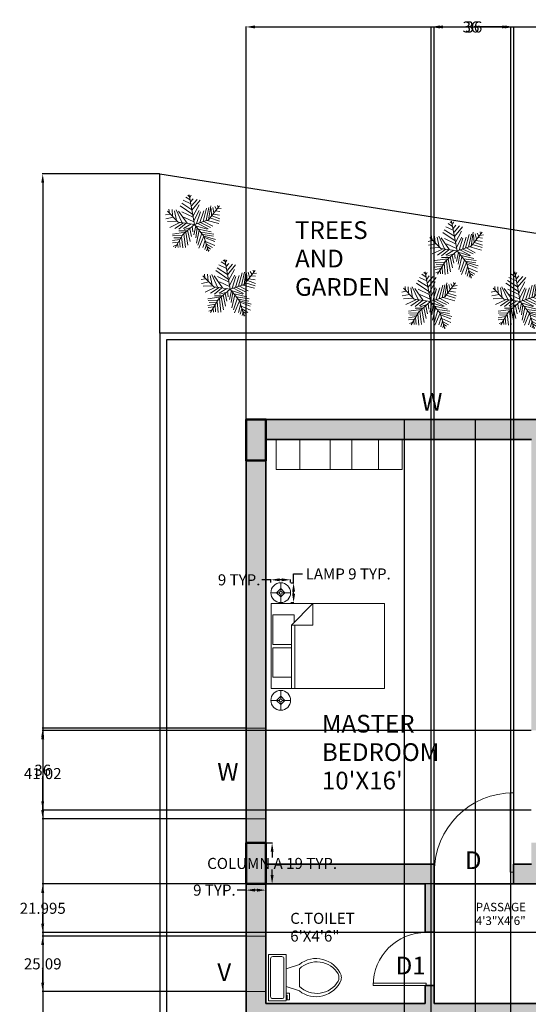
# Model space of a CAD drawing. Units: inches. Extents: x 460 to 1030, y -658 to 271.
# Tile 7 of 10: x 460 to 690, y -174 to 271. Entities that reach past the tile are written whole.
import ezdxf

# ---------------------------------------------------------------- set-up
doc = ezdxf.new("R2010")
doc.units = ezdxf.units.IN
doc.header["$MEASUREMENT"] = 0
for name, color, linetype, lineweight in [('A-ANNO-DIMS', 2, 'Continuous', 18), ('A-ANNO-TEXT', 7, 'Continuous', 18), ('A-AREA-IDEN', 7, 'Continuous', 25), ('A-COLS', 7, 'Continuous', 50), ('A-DOOR', 3, 'Continuous', 20), ('A-FLOR-CASE', 9, 'Continuous', 18), ('A-FLOR-FIXT', 9, 'Continuous', 18), ('A-FURN', 8, 'Continuous', 18), ('A-GLAZ', 4, 'Continuous', 20), ('A-GLAZ-PATT', 4, 'Continuous', 13), ('A-WALL', 7, 'Continuous', 35), ('A-WALL-PATT', 5, 'Continuous', 13), ('C-ANNO-TEXT', 7, 'Continuous', 18), ('C-PROP', 7, 'Continuous', 25), ('L-PLNT', 94, 'Continuous', 13)]:
    doc.layers.add(name, color=color, linetype=linetype, lineweight=lineweight)
doc.layers.add('A-COLS-PATT', color=7, linetype='Continuous', lineweight=13, true_color=0xffffff)
doc.styles.get("Standard").update_dxf_attribs({"font": 'arial.ttf'})
doc.dimstyles.get("Standard").update_dxf_attribs({"dimtxt": 5, "dimasz": 4, "dimexe": 0.18, "dimexo": 0.0625, "dimgap": 0.09, "dimtad": 0, "dimtih": 1, "dimtoh": 1, "dimdec": 1, "dimzin": 0, "dimdsep": 46, "dimlunit": 4, "dimtxsty": 'Standard', "dimcen": 0.09, "dimadec": 0, "dimazin": 0, "dimtfac": 1, "dimtdec": 1, "dimtofl": 0, "dimtmove": 0, "dimatfit": 3, "dimfxl": 1, "dimtolj": 1, "dimtzin": 0, "dimarcsym": 0})

# ---------------------------------------------------------------- blocks, each defined once
blk = doc.blocks.new('Bed - Queen')
for p, q in [((0, -80.00003), (0, 0)), ((0, 0), (59.99999, 0)), ((59.99999, 0), (59.99999, -80.00003)), ((7.99999, -1.2), (28.79998, -1.2)), ((7.99999, -14.4), (7.99999, -1.2)), ((28.79998, -1.2), (28.79998, -14.4)), ((31.19999, -1.2), (51.99999, -1.2)), ((31.19999, -14.4), (31.19999, -1.2)), ((51.99999, -1.2), (51.99999, -16.4)), ((0, -14.4), (44.8, -14.4)), ((44.8, -16.8), (0, -16.8)), ((59.99999, -29.6), (44.8, -14.4)), ((44.8, -14.4), (44.8, -29.6)), ((51.99999, -16.4), (46.79936, -16.4)), ((44.8, -29.6), (59.99999, -29.6)), ((59.99999, -80.00003), (0, -80.00003))]:
    blk.add_line(p, q)
blk = doc.blocks.new('Lamp - Table')
for p, q in [((0, 7), (0, 1)), ((-1, 0), (-7, 0)), ((0, 3), (-3, 0)), ((-3, 0), (0, -3)), ((3, 0), (0, 3)), ((0, -3), (3, 0)), ((1, 0), (7, 0)), ((0, -1), (0, -7))]:
    blk.add_line(p, q)
for radius in [7, 1]:
    blk.add_circle((0, 0), radius)
blk = doc.blocks.new('*U2')
for p, q in [((0, 0), (0, -6)), ((40, 0), (40, -6))]:
    blk.add_line(p, q)
blk.add_lwpolyline([(0, 0), (0, 40), (1.75, 40), (1.75, 0)], close=True)
blk.add_arc((0, 0), 40, 0, 90)
blk = doc.blocks.new('*U4')
for p, q in [((9.5, -6), (9.5, -2)), ((-10, -8.5), (-8, -8.5)), ((-10, -9.5), (-10, -8.5)), ((-8, -8.5), (-8, -8)), ((-7, -8), (-7, -9.5)), ((-4, -8), (-6, -14)), ((4, -8), (6, -14)), ((-7, -9.5), (-10, -9.5)), ((4, -14), (-4, -14))]:
    blk.add_line(p, q)
blk.add_lwpolyline([(10.5, -8), (10.5, 0), (-10.5, 0), (-10.5, -8)], close=True)
for points in [[(-9.5, -2), (-9.5, -6)], [(8.5, -1), (-8.5, -1)], [(-8.5, -7), (8.5, -7)]]:
    blk.add_lwpolyline(points)
for centre, radius, start, end in [((-8.62, -1.88), 0.884, 81.8699, 188.1301), ((8.62, -1.88), 0.884, 351.8699, 98.1301), ((-8.62, -6.12), 0.884, 171.8699, 278.1301), ((8.62, -6.12), 0.884, 261.8699, 8.1301), ((3.52, -21.58), 12.17, 141.4691, 247.9714), ((4.2, -21.82), 11.33, 136.3677, 238.9468), ((-3.52, -21.58), 12.17, 292.0284, 38.5307), ((-4.2, -21.82), 11.33, 301.053, 43.6321), ((0, -27.88), 4, 245.7318, 294.2682), ((0, -29), 4, 254.8605, 285.1395)]:
    blk.add_arc(centre, radius, start, end)
blk = doc.blocks.new('*U11')
for p, q in [((0, 0), (-266.7, 1447.8)), ((-129.8956, 713.6638), (-626.7704, 1032.1544)), ((-185.1152, 1008.5578), (-553.1612, 1185.4942)), ((-221.9198, 1197.3052), (-433.5526, 1338.8594)), ((-258.7244, 1362.456), (-332.3336, 1421.4348)), ((-231.1146, 1315.2628), (-166.7002, 1421.4348)), ((-194.31, 1102.9442), (-65.4812, 1256.284)), ((-148.3106, 914.1968), (118.5418, 1220.9018)), ((-129.8956, 701.8528), (265.7602, 1185.4942)), ((-1206.4492, 501.3198), (-1418.082, 465.9376)), ((-800.1, 114.3), (-1333.5, 647.7)), ((-1234.059, 536.7274), (-1252.4486, 737.2604)), ((-1105.2302, 725.4494), (-1077.6458, 395.1732)), ((-976.4268, 666.4706), (-884.4026, 194.6402)), ((-902.8176, 713.6638), (-617.5756, 100.2538)), ((-369.1382, 53.086), (-783.1836, 642.874)), ((-93.091, 489.5342), (-700.3796, 902.3858)), ((-617.5756, 607.4918), (-74.7014, 347.98)), ((-74.7014, 418.7444), (219.7608, 961.39)), ((-28.6766, 171.0436), (228.9556, 678.2816)), ((100.1268, 41.275), (284.1498, 619.2774)), ((256.5654, 88.4682), (449.7832, 666.4706)), ((412.9786, 147.447), (587.8068, 796.2392)), ((560.197, 182.8292), (698.2206, 819.8358)), ((685.8, 228.6), (1219.2, 914.4)), ((689.0258, 230.0224), (790.2448, 914.1968)), ((808.6344, 784.4282), (827.0494, 418.7444)), ((891.4384, 831.6214), (946.658, 572.1096)), ((919.0482, 501.3198), (1222.6798, 454.152)), ((983.4626, 867.0036), (1066.2666, 725.4494)), ((1029.462, 654.685), (1241.0948, 631.0884)), ((1112.2914, 760.8316), (1296.3144, 784.4282)), ((1121.4862, 925.9824), (1149.0706, 831.6214)), ((-1031.621, 347.98), (-1399.667, 277.1902)), ((-847.598, 159.2326), (-1326.0578, 135.636)), ((-718.7946, 88.4682), (-1215.644, -147.447)), ((-543.9664, 76.6572), (-967.2066, -206.4512)), ((0, 0), (-800.1, 114.3)), ((-405.9428, 53.086), (-764.794, -241.8334)), ((0, 0), (-571.5, -495.3)), ((-166.7002, 29.4894), (-543.9664, -206.4512)), ((-525.5514, 347.98), (-28.6766, 123.8504)), ((0, 0), (685.8, 228.6)), ((0, 0), (457.2, -571.5)), ((164.5412, 41.275), (661.416, -218.2368)), ((284.1498, 88.4682), (781.0246, -147.447)), ((458.978, 147.447), (891.4384, -88.4682)), ((615.4166, 194.6402), (1185.8752, 41.275)), ((753.4148, 312.5978), (1222.6798, 159.2326)), ((845.439, 418.7444), (1241.0948, 277.1902)), ((-442.7474, -383.3876), (-1086.8406, -477.7486)), ((-387.5278, -324.4088), (-764.794, -324.4088)), ((-525.5514, -465.963), (-451.9422, -1126.5408)), ((-166.7002, -147.447), (-507.1618, -253.619)), ((-433.5526, -383.3876), (-323.1134, -1020.3688)), ((-341.5284, -289.0012), (-221.9198, -831.6214)), ((-240.3094, -218.2368), (-157.5054, -595.7062)), ((-120.7008, -88.4682), (-93.091, -371.5766)), ((63.3222, -76.6826), (-37.8714, -513.1308)), ((44.9326, -64.897), (615.4166, -241.8334)), ((127.7366, -159.258), (54.1274, -654.685)), ((228.9556, -289.0012), (90.932, -914.1968)), ((357.759, -430.5554), (164.5412, -1020.3688)), ((192.151, -230.0224), (817.8292, -371.5766)), ((311.7596, -383.3876), (937.4378, -477.7486)), ((-718.7946, -737.2604), (-1086.8406, -796.2392)), ((-617.5756, -548.5384), (-1077.6458, -560.324)), ((-783.1836, -867.029), (-1077.6458, -902.4112)), ((-681.9646, -666.496), (-1022.4262, -654.685)), ((-571.5, -495.3), (-952.5, -1143)), ((-829.2084, -937.7934), (-810.7934, -1126.5408)), ((-737.1842, -784.4536), (-709.5744, -1114.7298)), ((-635.9652, -607.5172), (-580.771, -1150.1374)), ((458.978, -572.1096), (210.5406, -1161.923)), ((514.1976, -772.6426), (403.7838, -1138.3264)), ((412.9786, -501.3452), (919.0482, -583.9206)), ((457.2, -571.5), (685.8, -1333.5)), ((468.1982, -572.1096), (1029.462, -737.2604)), ((486.5878, -642.8994), (983.4626, -843.4324)), ((578.612, -961.39), (495.7826, -1232.7128)), ((541.8074, -831.6214), (992.6574, -1032.1544)), ((-875.2078, -1008.5832), (-1040.8412, -1079.3476)), ((578.612, -973.1756), (873.0488, -1138.3264)), ((624.6114, -1161.923), (587.8068, -1291.6916)), ((624.6114, -1102.9442), (781.0246, -1209.1162)), ((679.8056, -1268.095), (716.6102, -1291.6916))]:
    blk.add_line(p, q)
blk = doc.blocks.new('BEDROOM-STORAGE-UNIT')
for p, q in [((10.68, 0), (10.68, -13.59)), ((24.45, 0), (24.45, -13.59)), ((34.21, 0), (34.21, -13.59)), ((46.22, 0), (46.22, -13.59))]:
    blk.add_line(p, q)
blk.add_lwpolyline([(0, 0), (57.01, 0), (57.01, -13.59), (0, -13.59)], close=True)
blk = doc.blocks.new('COL-RECT-TYPE-A')
blk.add_lwpolyline([(0, 0), (9, 0), (9, -18.58), (0, -18.58)], close=True)
blk = doc.blocks.new('*D19')
at = {"layer": 'A-ANNO-DIMS', "color": 0, "lineweight": -2, "transparency": 16777216}
for p, q in [((571.86, -101.15), (574.76, -101.15)), ((574.58, -105.15), (574.58, -107.76)), ((574.58, -115.73), (574.58, -113.11)), ((571.86, -119.73), (574.76, -119.73))]:
    blk.add_line(p, q, dxfattribs=at)
at = {"layer": 'A-ANNO-DIMS', "color": 0, "transparency": 16777216}
for points in [[(573.92, -105.15), (575.25, -105.15), (574.58, -101.15)], [(573.92, -115.73), (575.25, -115.73), (574.58, -119.73)]]:
    blk.add_solid(points, dxfattribs=at)
at = {"layer": 'Defpoints', "color": 0, "transparency": 16777216}
for p in [(571.8, -101.15), (571.8, -119.73), (574.58, -119.73)]:
    blk.add_point(p, dxfattribs=at)
at = {"layer": 'A-ANNO-DIMS', "color": 0, "transparency": 16777216, "insert": (574.58, -110.44), "char_height": 5, "attachment_point": 5}
blk.add_mtext('\\A1;COLUMN A 19 TYP.', dxfattribs=at)
blk = doc.blocks.new('*D20')
at = {"layer": 'A-ANNO-DIMS', "color": 0, "lineweight": -2, "transparency": 16777216}
for p, q in [((562.8, -119.79), (562.8, -122.69)), ((571.8, -119.79), (571.8, -122.69)), ((562.8, -122.51), (558.8, -122.51)), ((567.8, -122.51), (566.8, -122.51))]:
    blk.add_line(p, q, dxfattribs=at)
at = {"layer": 'A-ANNO-DIMS', "color": 0, "transparency": 16777216}
for points in [[(566.8, -121.85), (566.8, -123.18), (562.8, -122.51)], [(567.8, -121.85), (567.8, -123.18), (571.8, -122.51)]]:
    blk.add_solid(points, dxfattribs=at)
at = {"layer": 'Defpoints', "color": 0, "transparency": 16777216}
for p in [(562.8, -119.73), (571.8, -119.73), (562.8, -122.51)]:
    blk.add_point(p, dxfattribs=at)
at = {"layer": 'A-ANNO-DIMS', "color": 0, "transparency": 16777216, "insert": (548.48, -122.51), "char_height": 5, "attachment_point": 5}
blk.add_mtext('\\A1;9 TYP.', dxfattribs=at)
blk = doc.blocks.new('*D23')
at = {"layer": 'A-ANNO-DIMS', "color": 0, "lineweight": -2, "transparency": 16777216}
for p, q in [((584.29, 16.44), (584.29, 20.44)), ((584.29, 20.44), (588.29, 20.44)), ((583.01, 16.44), (584.47, 16.44)), ((584.29, 11.48), (584.29, 12.44)), ((583.01, 7.48), (584.47, 7.48))]:
    blk.add_line(p, q, dxfattribs=at)
at = {"layer": 'A-ANNO-DIMS', "color": 0, "transparency": 16777216}
for points in [[(583.63, 12.44), (584.96, 12.44), (584.29, 16.44)], [(583.63, 11.48), (584.96, 11.48), (584.29, 7.48)]]:
    blk.add_solid(points, dxfattribs=at)
at = {"layer": 'Defpoints', "color": 0, "transparency": 16777216}
for p in [(582.95, 16.44), (584.29, 16.44), (582.95, 7.48)]:
    blk.add_point(p, dxfattribs=at)
at = {"layer": 'A-ANNO-DIMS', "color": 0, "transparency": 16777216, "insert": (608.98, 20.44), "char_height": 5, "attachment_point": 5}
blk.add_mtext('\\A1;LAMP 9 TYP.', dxfattribs=at)
blk = doc.blocks.new('*D24')
at = {"layer": 'A-ANNO-DIMS', "color": 0, "lineweight": -2, "transparency": 16777216}
for p, q in [((573.99, 16.5), (573.99, 17.96)), ((582.95, 16.5), (582.95, 17.96)), ((573.99, 17.78), (569.99, 17.78)), ((578.95, 17.78), (577.99, 17.78))]:
    blk.add_line(p, q, dxfattribs=at)
at = {"layer": 'A-ANNO-DIMS', "color": 0, "transparency": 16777216}
for points in [[(577.99, 18.45), (577.99, 17.12), (573.99, 17.78)], [(578.95, 18.45), (578.95, 17.12), (582.95, 17.78)]]:
    blk.add_solid(points, dxfattribs=at)
at = {"layer": 'Defpoints', "color": 0, "transparency": 16777216}
for p in [(573.99, 17.78), (573.99, 16.44), (582.95, 16.44)]:
    blk.add_point(p, dxfattribs=at)
at = {"layer": 'A-ANNO-DIMS', "color": 0, "transparency": 16777216, "insert": (559.67, 17.78), "char_height": 5, "attachment_point": 5}
blk.add_mtext('\\A1;9 TYP.', dxfattribs=at)
blk = doc.blocks.new('*D40')
at = {"layer": 'A-ANNO-DIMS', "color": 0, "lineweight": -2, "transparency": 16777216}
for p, q in [((523.73, 201.27), (470.68, 201.27)), ((470.86, 197.27), (470.86, -202.58)), ((470.86, -607.73), (470.86, -207.87)), ((523.73, -611.73), (470.68, -611.73))]:
    blk.add_line(p, q, dxfattribs=at)
at = {"layer": 'A-ANNO-DIMS', "color": 0, "transparency": 16777216}
for points in [[(470.19, 197.27), (471.52, 197.27), (470.86, 201.27)], [(470.19, -607.73), (471.52, -607.73), (470.86, -611.73)]]:
    blk.add_solid(points, dxfattribs=at)
at = {"layer": 'Defpoints', "color": 0, "transparency": 16777216}
for p in [(470.86, 201.27), (523.8, 201.27), (523.8, -611.73)]:
    blk.add_point(p, dxfattribs=at)
at = {"layer": 'A-ANNO-DIMS', "color": 0, "transparency": 16777216, "insert": (470.86, -205.23), "char_height": 5, "attachment_point": 5}
blk.add_mtext('\\A1;813', dxfattribs=at)
blk = doc.blocks.new('*D43')
at = {"layer": 'A-ANNO-DIMS', "color": 0, "lineweight": -2, "transparency": 16777216}
for p, q in [((562.8, 90.34), (562.8, 267.89)), ((566.8, 267.71), (746.18, 267.71)), ((936.8, 267.71), (757.41, 267.71)), ((940.8, 90.34), (940.8, 267.89))]:
    blk.add_line(p, q, dxfattribs=at)
at = {"layer": 'A-ANNO-DIMS', "color": 0, "transparency": 16777216}
for points in [[(566.8, 268.38), (566.8, 267.04), (562.8, 267.71)], [(936.8, 268.38), (936.8, 267.04), (940.8, 267.71)]]:
    blk.add_solid(points, dxfattribs=at)
at = {"layer": 'Defpoints', "color": 0, "transparency": 16777216}
for p in [(940.8, 267.71), (562.8, 90.27), (940.8, 90.27)]:
    blk.add_point(p, dxfattribs=at)
at = {"layer": 'A-ANNO-DIMS', "color": 0, "transparency": 16777216, "insert": (751.8, 267.71), "char_height": 5, "attachment_point": 5}
blk.add_mtext('\\A1;378', dxfattribs=at)
blk = doc.blocks.new('*D55')
at = {"layer": 'A-ANNO-DIMS', "color": 0, "lineweight": -2, "transparency": 16777216}
for p, q in [((894.56, -119.73), (470.68, -119.73)), ((470.86, -123.73), (470.86, -128.08)), ((470.86, -137.72), (470.86, -133.37)), ((894.55, -141.72), (470.68, -141.72))]:
    blk.add_line(p, q, dxfattribs=at)
at = {"layer": 'A-ANNO-DIMS', "color": 0, "transparency": 16777216}
for points in [[(470.19, -123.73), (471.52, -123.73), (470.86, -119.73)], [(470.19, -137.72), (471.52, -137.72), (470.86, -141.72)]]:
    blk.add_solid(points, dxfattribs=at)
at = {"layer": 'Defpoints', "color": 0, "transparency": 16777216}
for p in [(470.86, -119.73), (894.62, -119.73), (894.61, -141.72)]:
    blk.add_point(p, dxfattribs=at)
at = {"layer": 'A-ANNO-DIMS', "color": 0, "transparency": 16777216, "insert": (470.86, -130.72), "char_height": 5, "attachment_point": 5}
blk.add_mtext('\\A1;21.995', dxfattribs=at)
blk = doc.blocks.new('*D56')
at = {"layer": 'A-ANNO-DIMS', "color": 0, "lineweight": -2, "transparency": 16777216}
for p, q in [((647.8, -110.66), (647.8, 267.89)), ((651.8, 267.71), (662.13, 267.71)), ((679.8, 267.71), (669.46, 267.71)), ((683.8, -110.66), (683.8, 267.89))]:
    blk.add_line(p, q, dxfattribs=at)
at = {"layer": 'A-ANNO-DIMS', "color": 0, "transparency": 16777216}
for points in [[(651.8, 268.38), (651.8, 267.04), (647.8, 267.71)], [(679.8, 268.38), (679.8, 267.04), (683.8, 267.71)]]:
    blk.add_solid(points, dxfattribs=at)
at = {"layer": 'Defpoints', "color": 0, "transparency": 16777216}
for p in [(683.8, 267.71), (647.8, -110.73), (683.8, -110.73)]:
    blk.add_point(p, dxfattribs=at)
at = {"layer": 'A-ANNO-DIMS', "color": 0, "transparency": 16777216, "insert": (665.8, 267.71), "char_height": 5, "attachment_point": 5}
blk.add_mtext('\\A1;36', dxfattribs=at)
blk = doc.blocks.new('*D58')
at = {"layer": 'A-ANNO-DIMS', "color": 0, "lineweight": -2, "transparency": 16777216}
for p, q in [((691.73, -50.3), (470.68, -50.3)), ((470.86, -54.3), (470.86, -65.65)), ((470.86, -82.3), (470.86, -70.94)), ((691.73, -86.3), (470.68, -86.3))]:
    blk.add_line(p, q, dxfattribs=at)
at = {"layer": 'A-ANNO-DIMS', "color": 0, "transparency": 16777216}
for points in [[(470.19, -54.3), (471.52, -54.3), (470.86, -50.3)], [(470.19, -82.3), (471.52, -82.3), (470.86, -86.3)]]:
    blk.add_solid(points, dxfattribs=at)
at = {"layer": 'Defpoints', "color": 0, "transparency": 16777216}
for p in [(691.8, -50.3), (470.86, -86.3), (691.8, -86.3)]:
    blk.add_point(p, dxfattribs=at)
at = {"layer": 'A-ANNO-DIMS', "color": 0, "transparency": 16777216, "insert": (470.86, -68.3), "char_height": 5, "attachment_point": 5}
blk.add_mtext('\\A1;36', dxfattribs=at)
blk = doc.blocks.new('*D61')
at = {"layer": 'A-ANNO-DIMS', "color": 0, "lineweight": -2, "transparency": 16777216}
for p, q in [((646.47, -287.66), (646.47, 267.89)), ((650.47, 267.71), (660.81, 267.71)), ((678.47, 267.71), (668.14, 267.71)), ((682.47, -287.66), (682.47, 267.89))]:
    blk.add_line(p, q, dxfattribs=at)
at = {"layer": 'A-ANNO-DIMS', "color": 0, "transparency": 16777216}
for points in [[(650.47, 268.38), (650.47, 267.04), (646.47, 267.71)], [(678.47, 268.38), (678.47, 267.04), (682.47, 267.71)]]:
    blk.add_solid(points, dxfattribs=at)
at = {"layer": 'Defpoints', "color": 0, "transparency": 16777216}
for p in [(682.47, 267.71), (646.47, -287.73), (682.47, -287.73)]:
    blk.add_point(p, dxfattribs=at)
at = {"layer": 'A-ANNO-DIMS', "color": 0, "transparency": 16777216, "insert": (664.47, 267.71), "char_height": 5, "attachment_point": 5}
blk.add_mtext('\\A1;36', dxfattribs=at)
blk = doc.blocks.new('*D68')
at = {"layer": 'A-ANNO-DIMS', "color": 0, "lineweight": -2, "transparency": 16777216}
for p, q in [((634.27, 90.21), (634.27, -654.61)), ((666.46, 90.21), (666.46, -654.61)), ((638.27, -654.43), (639.91, -654.43)), ((662.46, -654.43), (660.82, -654.43))]:
    blk.add_line(p, q, dxfattribs=at)
at = {"layer": 'A-ANNO-DIMS', "color": 0, "transparency": 16777216}
for points in [[(638.27, -653.77), (638.27, -655.1), (634.27, -654.43)], [(662.46, -653.77), (662.46, -655.1), (666.46, -654.43)]]:
    blk.add_solid(points, dxfattribs=at)
at = {"layer": 'Defpoints', "color": 0, "transparency": 16777216}
for p in [(634.27, 90.27), (666.46, 90.27), (666.46, -654.43)]:
    blk.add_point(p, dxfattribs=at)
at = {"layer": 'A-ANNO-DIMS', "color": 0, "transparency": 16777216, "insert": (650.37, -654.43), "char_height": 5, "attachment_point": 5}
blk.add_mtext('\\A1;32.184', dxfattribs=at)
blk = doc.blocks.new('*D74')
at = {"layer": 'A-ANNO-DIMS', "color": 0, "lineweight": -2, "transparency": 16777216}
for p, q in [((562.73, -49.3), (470.68, -49.3)), ((470.86, -53.3), (470.86, -67.17)), ((470.86, -86.32), (470.86, -72.45)), ((562.73, -90.32), (470.68, -90.32))]:
    blk.add_line(p, q, dxfattribs=at)
at = {"layer": 'A-ANNO-DIMS', "color": 0, "transparency": 16777216}
for points in [[(470.19, -53.3), (471.52, -53.3), (470.86, -49.3)], [(470.19, -86.32), (471.52, -86.32), (470.86, -90.32)]]:
    blk.add_solid(points, dxfattribs=at)
at = {"layer": 'Defpoints', "color": 0, "transparency": 16777216}
for p in [(562.8, -49.3), (470.86, -90.32), (562.8, -90.32)]:
    blk.add_point(p, dxfattribs=at)
at = {"layer": 'A-ANNO-DIMS', "color": 0, "transparency": 16777216, "insert": (470.86, -69.81), "char_height": 5, "attachment_point": 5}
blk.add_mtext('\\A1;41.02', dxfattribs=at)
blk = doc.blocks.new('*D75')
at = {"layer": 'A-ANNO-DIMS', "color": 0, "lineweight": -2, "transparency": 16777216}
for p, q in [((562.73, -143.29), (470.68, -143.29)), ((470.86, -147.29), (470.86, -153.19)), ((470.86, -164.38), (470.86, -158.48)), ((562.73, -168.38), (470.68, -168.38))]:
    blk.add_line(p, q, dxfattribs=at)
at = {"layer": 'A-ANNO-DIMS', "color": 0, "transparency": 16777216}
for points in [[(470.19, -147.29), (471.52, -147.29), (470.86, -143.29)], [(470.19, -164.38), (471.52, -164.38), (470.86, -168.38)]]:
    blk.add_solid(points, dxfattribs=at)
at = {"layer": 'Defpoints', "color": 0, "transparency": 16777216}
for p in [(562.8, -143.29), (470.86, -168.38), (562.8, -168.38)]:
    blk.add_point(p, dxfattribs=at)
at = {"layer": 'A-ANNO-DIMS', "color": 0, "transparency": 16777216, "insert": (470.86, -155.83), "char_height": 5, "attachment_point": 5}
blk.add_mtext('\\A1;25.09', dxfattribs=at)

msp = doc.modelspace()

# ---------------------------------------------------------------- hatches: boundary and pattern name
at = {"layer": 'A-COLS-PATT'}
h = msp.add_hatch(color=256, dxfattribs=at)
h.dxf.hatch_style = 1
h.paths.add_polyline_path([(571.7961, 90.2738), (562.7961, 90.2738), (562.7961, 71.6966), (571.7961, 71.6966)])
h.paths.add_polyline_path([(700.7961, 90.2738), (691.7961, 90.2738), (691.7961, 71.6966), (700.7961, 71.6966)])
h.paths.add_polyline_path([(811.7961, 90.2738), (802.7961, 90.2738), (802.7961, 71.6966), (811.7961, 71.6966)])
h.paths.add_polyline_path([(940.7961, 90.2738), (931.7961, 90.2738), (931.7961, 71.6966), (940.7961, 71.6966)])
h.paths.add_polyline_path([(940.7961, -101.149), (931.7961, -101.149), (931.7961, -119.7262), (940.7961, -119.7262)])
h.paths.add_polyline_path([(940.7961, -268.3723), (931.7961, -268.3723), (931.7961, -287.7262), (940.7961, -287.7262)])
h.paths.add_polyline_path([(803.0275, -281.7262), (789.8237, -281.7262), (789.8237, -287.7262), (803.0275, -287.7262)])
h.paths.add_polyline_path([(700.7961, -303.809), (691.7961, -303.809), (691.7961, -323.8443), (700.7961, -323.8443)])
h.paths.add_polyline_path([(571.7961, -303.809), (562.7961, -303.809), (562.7961, -323.8443), (571.7961, -323.8443)])
h.paths.add_polyline_path([(571.7961, -413.1453), (562.7961, -413.1453), (562.7961, -432.4659), (571.7961, -432.4659)])
h.paths.add_polyline_path([(571.7961, -101.149), (562.7961, -101.149), (562.7961, -119.7262), (571.7961, -119.7262)])
h.paths.add_polyline_path([(700.7961, -101.0985), (691.7961, -101.0985), (691.7961, -119.7262), (700.7961, -119.7262)])
h.paths.add_polyline_path([(811.7961, -101.149), (802.7961, -101.149), (802.7961, -119.7262), (811.7961, -119.7262)])
at = {"layer": 'A-GLAZ-PATT'}
h = msp.add_hatch(color=256, dxfattribs=at)
h.dxf.hatch_style = 1
h.paths.add_polyline_path([(571.7961, -343.9041), (562.7961, -343.9041), (562.7961, -384.3969), (571.7961, -384.3969)])
h.paths.add_polyline_path([(571.7961, -143.2895), (562.7961, -143.2895), (562.7961, -168.3798), (571.7961, -168.3798)])
h.paths.add_polyline_path([(571.7961, -49.2966), (562.7961, -49.2966), (562.7961, -90.3192), (571.7961, -90.3192)])
h.paths.add_polyline_path([(666.4584, 90.2738), (634.2742, 90.2738), (634.2742, 81.2738), (666.4584, 81.2738)])
h.paths.add_polyline_path([(742.1779, 90.2738), (713.201, 90.2738), (713.201, 81.2738), (742.1779, 81.2738)])
h.paths.add_polyline_path([(797.2395, 90.2738), (768.2626, 90.2738), (768.2626, 81.2738), (797.2395, 81.2738)])
h.paths.add_polyline_path([(918.7723, 90.2738), (881.2728, 90.2738), (881.2728, 81.2738), (918.7723, 81.2738)])
h.paths.add_polyline_path([(940.7961, -60.0042), (931.7961, -60.0042), (931.7961, -95.7262), (940.7961, -95.7262)])
h.paths.add_polyline_path([(940.7961, -163.6558), (931.7961, -163.6558), (931.7961, -230.2946), (940.7961, -230.2946)])
h.paths.add_polyline_path([(913.7961, -331.7262), (835.7961, -331.7262), (835.7961, -332.7262), (913.7961, -332.7262)])
h.paths.add_polyline_path([(871.4559, -281.7262), (831.4302, -281.7262), (831.4302, -287.7262), (871.4559, -287.7262)])
h.paths.add_polyline_path([(774.8576, -281.7262), (716.7073, -281.7262), (716.7073, -287.7262), (774.8576, -287.7262)])
at = {"layer": 'A-WALL-PATT'}
h = msp.add_hatch(color=256, dxfattribs=at)
h.dxf.hatch_style = 1
h.paths.add_polyline_path([(634.2742, 90.2738), (571.7961, 90.2738), (571.7961, 81.2738), (634.2742, 81.2738)])
h.paths.add_polyline_path([(691.7961, 90.2738), (666.4584, 90.2738), (666.4584, 81.2738), (691.7961, 81.2738)])
h.paths.add_polyline_path([(713.201, 90.2738), (700.7961, 90.2738), (700.7961, 81.2738), (713.201, 81.2738)])
h.paths.add_polyline_path([(748.7961, 90.2738), (742.1779, 90.2738), (742.1779, 81.2738), (748.7961, 81.2738)])
h.paths.add_polyline_path([(768.2626, 90.2738), (754.7961, 90.2738), (754.7961, 81.2738), (768.2626, 81.2738)])
h.paths.add_polyline_path([(802.7961, 90.2738), (797.2395, 90.2738), (797.2395, 81.2738), (802.7961, 81.2738)])
h.paths.add_polyline_path([(881.2728, 90.2738), (811.7961, 90.2738), (811.7961, 81.2738), (881.2728, 81.2738)])
h.paths.add_polyline_path([(931.7961, 90.2738), (918.7723, 90.2738), (918.7723, 81.2738), (931.7961, 81.2738)])
h.paths.add_polyline_path([(940.7961, 71.6966), (931.7961, 71.6966), (931.7961, -60.0042), (940.7961, -60.0042)])
h.paths.add_polyline_path([(940.7961, -95.7262), (931.7961, -95.7262), (931.7961, -101.149), (940.7961, -101.149)])
h.paths.add_polyline_path([(931.7961, -110.7262), (894.6225, -110.7262), (894.6225, -119.7262), (931.7961, -119.7262)])
h.paths.add_polyline_path([(858.6225, -110.7262), (811.7961, -110.7262), (811.7961, -119.7262), (858.6225, -119.7262)])
h.paths.add_polyline_path([(940.7961, -119.7262), (931.7961, -119.7262), (931.7961, -141.7212), (931.7961, -163.6558), (940.7961, -163.6558)])
h.paths.add_polyline_path([(940.7961, -230.2946), (931.7961, -230.2946), (931.7961, -268.3723), (940.7961, -268.3723)])
h.paths.add_polyline_path([(931.7961, -281.7262), (908.3452, -281.7262), (908.3452, -285.0181), (908.3452, -287.7262), (931.7961, -287.7262)])
h.paths.add_polyline_path([(831.4302, -281.7262), (803.0275, -281.7262), (803.0275, -287.7262), (808.7961, -287.7262), (808.7961, -339.7262), (811.7961, -339.7262), (811.7961, -287.7262), (831.4302, -287.7262)])
h.paths.add_polyline_path([(789.8237, -281.7262), (774.8576, -281.7262), (774.8576, -287.7262), (789.8237, -287.7262)])
h.paths.add_polyline_path([(716.7073, -281.7262), (700.7961, -281.7262), (700.7961, -271.1977), (691.7961, -271.1977), (691.7961, -281.7262), (682.4735, -281.7262), (682.4735, -287.7262), (691.7961, -287.7262), (691.7961, -303.809), (700.7961, -303.809), (700.7961, -287.7262), (716.7073, -287.7262)])
h.paths.add_polyline_path([(700.7961, -323.8443), (691.7961, -323.8443), (691.7961, -413.1453), (700.7961, -413.1453)])
h.paths.add_polyline_path([(940.7961, -287.7262), (937.7961, -287.7262), (937.7961, -339.7262), (940.7961, -339.7262)])
h.paths.add_polyline_path([(937.7961, -336.7262), (811.7961, -336.7262), (811.7961, -339.7262), (937.7961, -339.7262)])
h.paths.add_polyline_path([(835.7961, -329.7262), (811.7961, -329.7262), (811.7961, -332.7262), (835.7961, -332.7262)])
h.paths.add_polyline_path([(937.7961, -329.7262), (913.7961, -329.7262), (913.7961, -332.7262), (937.7961, -332.7262)])
h.paths.add_polyline_path([(691.7961, -419.7262), (681.4044, -419.7262), (681.4044, -428.7262), (691.7961, -428.7262)])
h.paths.add_polyline_path([(691.7961, -476.7262), (571.7961, -476.7262), (571.7961, -485.7262), (691.7961, -485.7262)])
h.paths.add_polyline_path([(571.7961, -465.0348), (568.223, -465.0348), (562.7961, -465.0348), (562.7961, -476.7262), (571.7961, -476.7262)])
h.paths.add_polyline_path([(571.7961, -432.4659), (562.7961, -432.4659), (562.7961, -441.1912), (571.7961, -441.1912)])
h.paths.add_polyline_path([(571.7961, -384.3969), (562.7961, -384.3969), (562.7961, -413.1453), (571.7961, -413.1453)])
h.paths.add_polyline_path([(571.7961, -323.8443), (562.7961, -323.8443), (562.7961, -343.9041), (571.7961, -343.9041)])
h.paths.add_polyline_path([(571.7961, -287.7262), (646.4735, -287.7262), (646.4735, -281.7262), (571.7961, -281.7262), (571.7961, -258.1542), (571.7961, -233.7262), (566.4164, -233.7262), (562.7961, -233.7262), (562.7961, -303.809), (571.7961, -303.809)])
h.paths.add_polyline_path([(571.7961, -179.7262), (691.7961, -179.7262), (691.7961, -197.5753), (700.7961, -197.5753), (700.7961, -173.7262), (647.7961, -173.7262), (647.7961, -165.5723), (643.7961, -165.5723), (643.7961, -173.7262), (571.7961, -173.7262), (571.7961, -168.3798), (562.7961, -168.3798), (562.7961, -197.7262), (571.7961, -197.7262)])
h.paths.add_polyline_path([(647.7961, -110.7262), (571.7961, -110.7262), (571.7961, -119.7262), (643.7961, -119.7262), (643.7961, -141.5723), (647.7961, -141.5723)])
h.paths.add_polyline_path([(691.7961, -110.7262), (683.7961, -110.7262), (683.7961, -114.3453), (683.7961, -119.7262), (691.7961, -119.7262)])
h.paths.add_polyline_path([(571.7961, -119.7262), (562.7961, -119.7262), (562.7961, -143.2895), (571.7961, -143.2895)])
h.paths.add_polyline_path([(571.7961, -90.3192), (562.7961, -90.3192), (562.7961, -101.149), (571.7961, -101.149)])
h.paths.add_polyline_path([(571.7961, 71.6966), (562.7961, 71.6966), (562.7961, -49.2966), (571.7961, -49.2966)])
h.paths.add_polyline_path([(700.7961, 71.6966), (691.7961, 71.6966), (691.7961, -50.298), (700.7961, -50.298)])
h.paths.add_polyline_path([(754.7961, 81.2738), (748.7961, 81.2738), (748.7961, -38.7262), (741.5908, -38.7262), (741.5908, -39.109), (741.5908, -42.7262), (748.7961, -42.7262), (748.7961, -110.7262), (754.7961, -110.7262), (754.7961, -42.7262), (773.6274, -42.7262), (773.6274, -38.7262), (754.7961, -38.7262)])
h.paths.add_polyline_path([(717.4759, -38.7262), (700.7961, -38.7262), (700.7961, -42.7262), (717.4759, -42.7262)])
h.paths.add_polyline_path([(811.7961, 71.6966), (802.7961, 71.6966), (802.7961, -50.298), (811.7961, -50.298)])
h.paths.add_polyline_path([(811.7961, -86.298), (806.4164, -86.298), (802.7961, -86.298), (802.7961, -101.149), (811.7961, -101.149)])

# ---------------------------------------------------------------- linework, layer by layer
at = {"layer": 'A-GLAZ'}
for points in [[(666.4584, 81.2738), (634.2742, 81.2738), (634.2742, 90.2738), (666.4584, 90.2738)], [(571.7961, -90.3192), (562.7961, -90.3192), (562.7961, -49.2966), (571.7961, -49.2966)], [(571.7961, -168.3798), (562.7961, -168.3798), (562.7961, -143.2895), (571.7961, -143.2895)]]:
    msp.add_lwpolyline(points, close=True, dxfattribs=at)
at = {"layer": 'A-WALL'}
for p, q in [((562.7961, 90.2738), (562.7961, -197.7262)), ((940.7961, 90.2738), (562.7961, 90.2738)), ((571.7961, 81.2738), (571.7961, -110.7262)), ((691.7961, 81.2738), (571.7961, 81.2738)), ((647.7961, -110.7262), (571.7961, -110.7262)), ((647.7961, -110.7262), (647.7961, -173.7262)), ((683.7961, -110.7262), (683.7961, -119.7262)), ((691.7961, -110.7262), (683.7961, -110.7262)), ((571.7961, -119.7262), (571.7961, -173.7262)), ((643.7961, -119.7262), (571.7961, -119.7262)), ((643.7961, -119.7262), (643.7961, -141.5723)), ((940.7961, -119.7262), (647.7961, -119.7262)), ((647.7961, -141.5723), (643.7961, -141.5723)), ((643.7961, -165.5723), (647.7961, -165.5723)), ((643.7961, -165.5723), (643.7961, -173.7262)), ((643.7961, -173.7262), (571.7961, -173.7262)), ((700.7961, -173.7262), (647.7961, -173.7262))]:
    msp.add_line(p, q, dxfattribs=at)
at = {"layer": 'C-PROP'}
for p, q in [((523.7961, 129.2738), (523.7961, 201.2738)), ((523.7961, 201.2738), (979.7961, 129.2738)), ((523.7961, 129.2738), (523.7961, -524.7262)), ((936.9757, 129.2738), (523.7961, 129.2738)), ((526.7961, 126.2738), (526.7961, -608.7262)), ((976.7961, 126.2738), (526.7961, 126.2738))]:
    msp.add_line(p, q, dxfattribs=at)

# ---------------------------------------------------------------- block references
at = {"layer": 'A-COLS'}
msp.add_blockref('COL-RECT-TYPE-A', (562.7961, 90.2738), dxfattribs=at)
at = {"layer": 'A-COLS', "rotation": 180}
msp.add_blockref('COL-RECT-TYPE-A', (571.7961, -119.7262), dxfattribs=at)
at = {"layer": 'A-DOOR', "xscale": -0.8968184486891608, "yscale": 0.8968184486891608, "zscale": 0.8968184486891608}
msp.add_blockref('*U2', (683.7961, -114.3453), dxfattribs=at)
at = {"layer": 'A-DOOR', "xscale": 0.5986785969564075, "yscale": 0.5986785969564075, "zscale": 0.5986785969564075, "rotation": 90.00000000000003}
msp.add_blockref('*U2', (644.204, -165.5723), dxfattribs=at)
at = {"layer": 'A-FLOR-CASE'}
msp.add_blockref('BEDROOM-STORAGE-UNIT', (576.4129, 81.2738), dxfattribs=at)
at = {"layer": 'A-FLOR-FIXT', "rotation": 89.99999999999999}
msp.add_blockref('*U4', (572.9063, -162.0596), dxfattribs=at)
at = {"layer": 'A-FURN', "xscale": 0.6401435689940156, "yscale": 0.6401435689940156, "zscale": 0.6401435689940156, "rotation": 90}
for name, p in [('Lamp - Table', (578.4675, 11.9594)), ('Bed - Queen', (574.1087, -31.3746)), ('Lamp - Table', (578.4675, -36.7055))]:
    msp.add_blockref(name, p, dxfattribs=at)
at = {"layer": 'L-PLNT', "xscale": 0.0092368434635362, "yscale": 0.0092368434635362, "zscale": 0.0092368434635362}
for p in [(539.521, 178.4638), (658.2251, 166.4713), (555.591, 149.2105), (646.2677, 143.5676), (686.7899, 143.5676)]:
    msp.add_blockref('*U11', p, dxfattribs=at)

# ---------------------------------------------------------------- texts
at = {"layer": 'A-ANNO-TEXT'}
for s, p in [('W', (641.9792, 94.254)), ('W', (549.7936, -73.0567)), ('D', (661.7296, -112.9833)), ('V', (549.7936, -163.5706)), ('D1', (630.4589, -160.5987))]:
    msp.add_text(s, height=8, dxfattribs=at).set_placement(p)
at = {"layer": 'A-AREA-IDEN'}
for s, height, p in [('MASTER', 8, (597.0747, -51.2655)), ('BEDROOM', 8, (597.0747, -64.1168)), ("10'X16'", 8, (597.0747, -76.9681)), ('PASSAGE', 3.84922, (666.648, -132.0827)), ('C.TOILET', 4.98699, (582.7888, -137.7511)), ('4\'3"X4\'6"', 3.84922, (666.648, -138.2661)), ('6\'X4\'6"', 4.98699, (582.7888, -145.7623))]:
    msp.add_text(s, height=height, dxfattribs=at).set_placement(p)
at = {"layer": 'C-ANNO-TEXT'}
for s, p in [('TREES ', (584.9386, 171.8627)), ('AND ', (584.9386, 159.0114)), ('GARDEN', (584.9386, 146.1601))]:
    msp.add_text(s, height=8, dxfattribs=at).set_placement(p)

# ---------------------------------------------------------------- dimensions: what is measured, and where the dimension line sits
at = {"layer": 'A-ANNO-DIMS'}
for base, p1, p2, override, picture, middle in [((940.7961, 267.7108), (562.7961, 90.2738), (940.7961, 90.2738), {"dimdec": 0, "dimlfac": 1, "dimrnd": 0, "dimzin": 0, "dimdsep": 46, "dimlunit": 2}, '*D43', (751.7961, 267.7108)), ((682.4735, 267.7108), (646.4735, -287.7262), (682.4735, -287.7262), {"dimdec": 0, "dimlfac": 1, "dimrnd": 0, "dimzin": 0, "dimdsep": 46, "dimlunit": 2}, '*D61', (664.4735, 267.7108)), ((683.7961, 267.7108), (647.7961, -110.7262), (683.7961, -110.7262), {"dimdec": 0, "dimlfac": 1, "dimrnd": 0, "dimzin": 0, "dimdsep": 46, "dimlunit": 2}, '*D56', (665.7961, 267.7108)), ((666.4584, -654.4339), (634.2742, 90.2738), (666.4584, 90.2738), {"dimdec": 3, "dimlfac": 1, "dimrnd": 0, "dimzin": 0, "dimdsep": 46, "dimlunit": 2}, '*D68', (650.3663, -654.4339))]:
    dim = msp.add_linear_dim(base=base, p1=p1, p2=p2, dimstyle='Standard', override=override, dxfattribs=at)
    dim.commit()
    dim.dimension.update_dxf_attribs({"geometry": picture, "text_midpoint": middle})
for base, p1, p2, override, picture, middle in [((470.8563, 201.2738), (523.7961, -611.7262), (523.7961, 201.2738), {"dimdec": 0, "dimlfac": 1, "dimrnd": 0, "dimzin": 0, "dimdsep": 46, "dimlunit": 2}, '*D40', (470.8563, -205.2262)), ((470.8563, -90.3192), (562.7961, -49.2966), (562.7961, -90.3192), {"dimdec": 2, "dimlfac": 1, "dimrnd": 0, "dimzin": 0, "dimdsep": 46, "dimlunit": 2}, '*D74', (470.8563, -69.8079)), ((470.8563, -86.298), (691.7961, -50.298), (691.7961, -86.298), {"dimdec": 0, "dimlfac": 1, "dimrnd": 0, "dimzin": 0, "dimdsep": 46, "dimlunit": 2}, '*D58', (470.8563, -68.298)), ((470.8563, -119.7262), (894.6132, -141.7212), (894.6225, -119.7262), {"dimdec": 3, "dimlfac": 1, "dimrnd": 0, "dimzin": 0, "dimdsep": 46, "dimlunit": 2}, '*D55', (470.8563, -130.7237)), ((470.8563, -168.3798), (562.7961, -143.2895), (562.7961, -168.3798), {"dimdec": 2, "dimlfac": 1, "dimrnd": 0, "dimzin": 0, "dimdsep": 46, "dimlunit": 2}, '*D75', (470.8563, -155.8347))]:
    dim = msp.add_linear_dim(base=base, p1=p1, p2=p2, angle=90, dimstyle='Standard', override=override, dxfattribs=at)
    dim.commit()
    dim.dimension.update_dxf_attribs({"geometry": picture, "text_midpoint": middle})
for base, p1, p2, angle, text, picture, middle in [((584.2928, 16.4404), (582.9485, 7.4783), (582.9485, 16.4404), 90, 'LAMP <> TYP.', '*D23', (608.9797, 20.4404)), ((573.9865, 17.7847), (582.9485, 16.4404), (573.9865, 16.4404), 180, '<> TYP.', '*D24', (559.6697, 17.7847)), ((574.5827, -119.7262), (571.7961, -101.149), (571.7961, -119.7262), 270, 'COLUMN A <> TYP.', '*D19', (574.5827, -110.4376)), ((562.7961, -122.5128), (571.7961, -119.7262), (562.7961, -119.7262), 180, '<> TYP.', '*D20', (548.4793, -122.5128))]:
    dim = msp.add_linear_dim(base=base, p1=p1, p2=p2, angle=angle, text=text, dimstyle='Standard', override={"dimdec": 0, "dimlfac": 1, "dimrnd": 0, "dimzin": 0, "dimdsep": 46, "dimlunit": 2}, dxfattribs=at)
    dim.commit()
    dim.dimension.update_dxf_attribs({"geometry": picture, "text_midpoint": middle})

doc.saveas('drawing.dxf')
